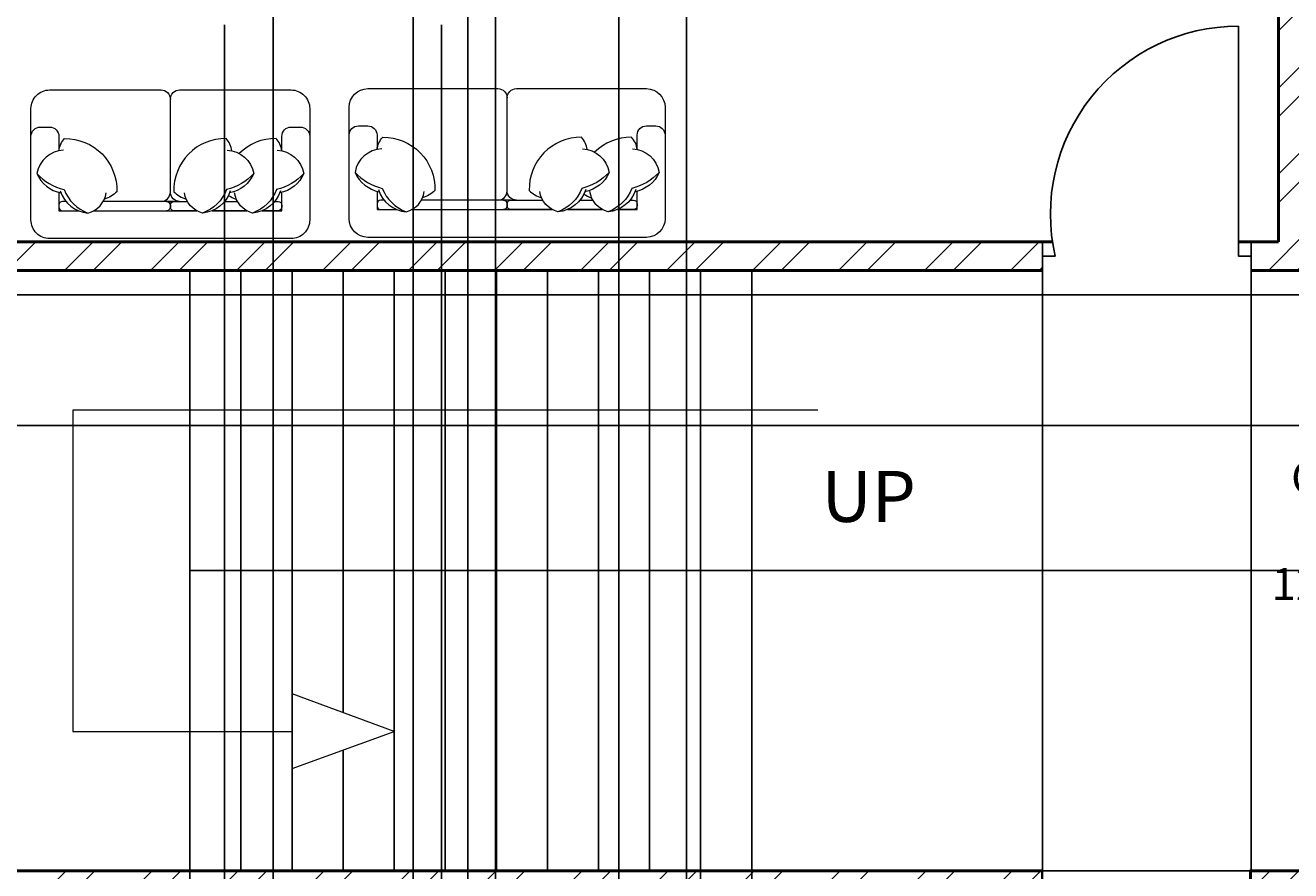
# Model space of a CAD drawing. Units: inches. Extents: x 2310 to 2937, y 1113 to 2410.
# Tile 8 of 23: x 2411 to 2609, y 2000 to 2132. Entities that reach past the tile are written whole.
import ezdxf

# ---------------------------------------------------------------- set-up
doc = ezdxf.new("R2010")
doc.units = ezdxf.units.IN
for name, color, linetype, lineweight in [('A-ANNO-DIMS', 2, 'Continuous', 18), ('A-ANNO-SYMB', 151, 'Continuous', 18), ('A-ANNO-TEXT', 7, 'Continuous', 18), ('A-AREA-IDEN', 7, 'Continuous', 18), ('A-DOOR', 31, 'Continuous', 25), ('A-FLOR-STRS', 151, 'Continuous', 25), ('A-FURN', 8, 'Continuous', 18), ('A-WALL', 7, 'Continuous', 50), ('A-WALL-PATT', 85, 'Continuous', 13)]:
    doc.layers.add(name, color=color, linetype=linetype, lineweight=lineweight)
doc.styles.get("Standard").update_dxf_attribs({"font": 'arial.ttf'})
doc.dimstyles.get("Standard").update_dxf_attribs({"dimtxt": 0.18, "dimasz": 0.18, "dimexe": 0.18, "dimexo": 0.0625, "dimgap": 0.09, "dimtad": 0, "dimtih": 1, "dimtoh": 1, "dimdec": 4, "dimzin": 0, "dimdsep": 46, "dimtxsty": 'Standard', "dimcen": 0.09, "dimadec": 0, "dimazin": 0, "dimtfac": 1, "dimtdec": 4, "dimtofl": 0, "dimtmove": 0, "dimatfit": 3, "dimfxl": 1, "dimtolj": 1, "dimtzin": 0, "dimarcsym": 0})

# ---------------------------------------------------------------- blocks, each defined once
blk = doc.blocks.new('SOFA-COMPACT')
at = {"ltscale": 0.03}
blk.add_lwpolyline([(20.37, 23.28, -0.414214), (21.83, 21.83, -0.414214), (23.28, 23.28), (40.75, 23.28, -0.414214), (43.66, 20.37), (43.66, 2.91, -0.414214), (40.75, 0), (2.91, 0, -0.414214), (0, 2.91), (0, 20.37, -0.414214), (2.91, 23.28), (20.37, 23.28, -0.414214), (21.83, 21.83, -0.414214), (23.28, 23.28)], format="xyb", dxfattribs=at)
for points in [[(20.37, 5.82, 0.414214), (21.83, 7.28), (21.83, 21.83, 0.414214)], [(23.28, 5.82, -0.414214), (21.83, 7.28), (21.83, 21.83, -0.414214)], [(0, 16.01, -0.414214), (1.46, 17.46), (2.91, 17.46, -0.414214), (4.37, 16.01), (4.37, 13.75)], [(39.29, 13.75), (39.29, 16.01, -0.414214), (40.75, 17.46), (42.2, 17.46, -0.414214), (43.66, 16.01)], [(4.36, 13.75, -0.165541), (5.26, 15.67, -0.425989), (13.44, 7.34, -0.121523), (11.5, 6.19, 7.115464)], [(31.45, 13.75, 0.165541), (30.55, 15.67, 0.425989), (22.38, 7.34, 0.121523), (24.32, 6.19, -7.115464)], [(39.29, 13.75, 0.165541), (38.39, 15.67, 0.200231), (32.62, 13.33, 0.121523)], [(5.1, 13.84, 0.356772), (0.93, 10.17, 0.249542), (4.7, 7.15, -9.61688)], [(30.72, 13.84, -0.356772), (34.89, 10.17, -0.249542), (31.11, 7.15, 9.61688)], [(38.56, 13.84, -0.356772), (42.73, 10.17, -0.249542), (38.95, 7.15, 9.61688)], [(0.93, 10.17, 0.14773), (5.18, 7.67, 0.213343), (8.93, 4, 0.178662)], [(34.89, 10.17, -0.14773), (30.64, 7.67, -0.213343), (26.88, 4, -0.178662)], [(42.73, 10.17, -0.14773), (38.48, 7.67, -0.213343), (34.72, 4, -0.178662)], [(4.59, 7.47, 0.306663), (8.93, 4, 0.30633), (11.77, 7.17, -0.872847)], [(20.37, 5.82, 0.414214), (21.83, 7.28)], [(23.28, 5.82, -0.414214), (21.83, 7.28)], [(31.22, 7.47, -0.306663), (26.88, 4, -0.30633), (24.05, 7.17, 0.872847)], [(30.94, 6.76, 0.071865), (32.16, 6.19, -7.115464)], [(39.06, 7.47, -0.306663), (34.72, 4, -0.30633), (31.89, 7.17, 0.872847)], [(36.23, 4.37), (39.29, 4.37), (39.29, 7.23, -0.414214)], [(5.48, 5.82), (4.95, 5.82, 0.414214), (4.37, 5.24), (4.37, 4.95, 0.414214), (4.95, 4.37)], [(4.95, 4.37), (7.43, 4.37, 0.414214)], [(9.85, 4.37), (21.25, 4.37, 0.414214), (21.83, 4.95), (21.83, 5.24, 0.414214), (21.25, 5.82), (11.31, 5.82, 0.414214)], [(25.97, 4.37), (22.41, 4.37, -0.414214), (21.83, 4.95), (21.83, 5.24, -0.414214), (22.41, 5.82), (24.5, 5.82, -0.414214)], [(33.81, 4.37), (28.39, 4.37, -0.414214)], [(30.34, 5.82), (32.34, 5.82, -0.414214)], [(38.71, 4.37), (36.23, 4.37, -0.414214)], [(38.18, 5.82), (38.71, 5.82, -0.414214), (39.29, 5.24), (39.29, 4.95, -0.414214), (38.71, 4.37)]]:
    blk.add_lwpolyline(points, format="xyb")
for points in [[(4.37, 7.23), (4.37, 4.37), (7.43, 4.37)], [(9.85, 4.37), (25.97, 4.37)], [(28.39, 4.37), (33.81, 4.37)]]:
    blk.add_lwpolyline(points)
blk.add_lwpolyline([(21.25, 4.37), (22.41, 4.37, -0.414214), (21.83, 4.95), (21.83, 5.24, -0.414214), (22.41, 5.82), (21.25, 5.82, -0.414214), (21.83, 5.24), (21.83, 4.95, -0.414214)], format="xyb", close=True)
blk = doc.blocks.new('*D41')
at = {"layer": 'A-ANNO-DIMS', "color": 0, "lineweight": -2, "transparency": 16777216}
for p, q in [((2479.99, 2347.45), (2479.99, 1649.5)), ((2503.66, 2347.45), (2503.66, 1649.5)), ((2480.17, 1649.68), (2491.36, 1649.68)), ((2503.48, 1649.68), (2492.29, 1649.68))]:
    blk.add_line(p, q, dxfattribs=at)
at = {"layer": 'A-ANNO-DIMS', "color": 0, "transparency": 16777216}
for points in [[(2480.17, 1649.71), (2480.17, 1649.65), (2479.99, 1649.68)], [(2503.48, 1649.71), (2503.48, 1649.65), (2503.66, 1649.68)]]:
    blk.add_solid(points, dxfattribs=at)
at = {"layer": 'Defpoints', "color": 0, "transparency": 16777216}
for p in [(2479.99, 2347.51), (2503.66, 2347.51), (2503.66, 1649.68)]:
    blk.add_point(p, dxfattribs=at)
at = {"layer": 'A-ANNO-DIMS', "color": 0, "transparency": 16777216, "insert": (2491.82, 1649.68), "char_height": 0.18, "attachment_point": 5}
blk.add_mtext('\\A1;23.676', dxfattribs=at)
blk = doc.blocks.new('*D60')
at = {"layer": 'A-ANNO-DIMS', "color": 0, "lineweight": -2, "transparency": 16777216}
for p, q in [((2449.5, 2205.95), (2449.5, 1649.5)), ((2471.44, 2205.95), (2471.44, 1649.5)), ((2449.68, 1649.68), (2460.01, 1649.68)), ((2471.26, 1649.68), (2460.94, 1649.68))]:
    blk.add_line(p, q, dxfattribs=at)
at = {"layer": 'A-ANNO-DIMS', "color": 0, "transparency": 16777216}
for points in [[(2449.68, 1649.71), (2449.68, 1649.65), (2449.5, 1649.68)], [(2471.26, 1649.71), (2471.26, 1649.65), (2471.44, 1649.68)]]:
    blk.add_solid(points, dxfattribs=at)
at = {"layer": 'Defpoints', "color": 0, "transparency": 16777216}
for p in [(2449.5, 2206.01), (2471.44, 2206.01), (2471.44, 1649.68)]:
    blk.add_point(p, dxfattribs=at)
at = {"layer": 'A-ANNO-DIMS', "color": 0, "transparency": 16777216, "insert": (2460.47, 1649.68), "char_height": 0.18, "attachment_point": 5}
blk.add_mtext('\\A1;21.936', dxfattribs=at)
blk = doc.blocks.new('*D61')
at = {"layer": 'A-ANNO-DIMS', "color": 0, "lineweight": -2, "transparency": 16777216}
for p, q in [((2484.33, 2205.95), (2484.33, 1649.5)), ((2514.27, 2205.95), (2514.27, 1649.5)), ((2484.51, 1649.68), (2498.9, 1649.68)), ((2514.09, 1649.68), (2499.69, 1649.68))]:
    blk.add_line(p, q, dxfattribs=at)
at = {"layer": 'A-ANNO-DIMS', "color": 0, "transparency": 16777216}
for points in [[(2484.51, 1649.71), (2484.51, 1649.65), (2484.33, 1649.68)], [(2514.09, 1649.71), (2514.09, 1649.65), (2514.27, 1649.68)]]:
    blk.add_solid(points, dxfattribs=at)
at = {"layer": 'Defpoints', "color": 0, "transparency": 16777216}
for p in [(2484.33, 2206.01), (2514.27, 2206.01), (2514.27, 1649.68)]:
    blk.add_point(p, dxfattribs=at)
at = {"layer": 'A-ANNO-DIMS', "color": 0, "transparency": 16777216, "insert": (2499.3, 1649.68), "char_height": 0.18, "attachment_point": 5}
blk.add_mtext('\\A1;29.94', dxfattribs=at)
blk = doc.blocks.new('*D62')
at = {"layer": 'A-ANNO-DIMS', "color": 0, "lineweight": -2, "transparency": 16777216}
for p, q in [((2569.99, 2093.45), (2569.99, 1649.5)), ((2602.69, 2093.45), (2602.69, 1649.5)), ((2570.17, 1649.68), (2586.02, 1649.68)), ((2602.51, 1649.68), (2586.66, 1649.68))]:
    blk.add_line(p, q, dxfattribs=at)
at = {"layer": 'A-ANNO-DIMS', "color": 0, "transparency": 16777216}
for points in [[(2570.17, 1649.71), (2570.17, 1649.65), (2569.99, 1649.68)], [(2602.51, 1649.71), (2602.51, 1649.65), (2602.69, 1649.68)]]:
    blk.add_solid(points, dxfattribs=at)
at = {"layer": 'Defpoints', "color": 0, "transparency": 16777216}
for p in [(2569.99, 2093.51), (2602.69, 2093.51), (2602.69, 1649.68)]:
    blk.add_point(p, dxfattribs=at)
at = {"layer": 'A-ANNO-DIMS', "color": 0, "transparency": 16777216, "insert": (2586.34, 1649.68), "char_height": 0.18, "attachment_point": 5}
blk.add_mtext('\\A1;32.7', dxfattribs=at)
blk = doc.blocks.new('*D64')
at = {"layer": 'A-ANNO-DIMS', "color": 0, "lineweight": -2, "transparency": 16777216}
for p, q in [((2524.527191, 2046.513944), (2858.015941, 2046.513944)), ((2857.835941, 2046.333944), (2857.835941, 2023.193944)), ((2857.835941, 1999.693944), (2857.835941, 2022.833944)), ((2524.527191, 1999.513944), (2858.015941, 1999.513944))]:
    blk.add_line(p, q, dxfattribs=at)
at = {"layer": 'A-ANNO-DIMS', "color": 0, "transparency": 16777216}
for points in [[(2857.805941, 2046.333944), (2857.865941, 2046.333944), (2857.835941, 2046.513944)], [(2857.805941, 1999.693944), (2857.865941, 1999.693944), (2857.835941, 1999.513944)]]:
    blk.add_solid(points, dxfattribs=at)
at = {"layer": 'Defpoints', "color": 0, "transparency": 16777216}
for p in [(2524.464691, 2046.513944), (2857.835941, 2046.513944), (2524.464691, 1999.513944)]:
    blk.add_point(p, dxfattribs=at)
at = {"layer": 'A-ANNO-DIMS', "color": 0, "transparency": 16777216, "insert": (2857.835941, 2023.013944), "char_height": 0.18, "attachment_point": 5}
blk.add_mtext('\\A1;47', dxfattribs=at)
blk = doc.blocks.new('*D65')
at = {"layer": 'A-ANNO-DIMS', "color": 0, "lineweight": -2, "transparency": 16777216}
for p, q in [((2403.49, 2093.45), (2403.49, 1649.5)), ((2436.46, 2093.45), (2436.46, 1649.5)), ((2403.67, 1649.68), (2419.58, 1649.68)), ((2436.28, 1649.68), (2420.37, 1649.68))]:
    blk.add_line(p, q, dxfattribs=at)
at = {"layer": 'A-ANNO-DIMS', "color": 0, "transparency": 16777216}
for points in [[(2403.67, 1649.71), (2403.67, 1649.65), (2403.49, 1649.68)], [(2436.28, 1649.71), (2436.28, 1649.65), (2436.46, 1649.68)]]:
    blk.add_solid(points, dxfattribs=at)
at = {"layer": 'Defpoints', "color": 0, "transparency": 16777216}
for p in [(2403.49, 2093.51), (2436.46, 2093.51), (2436.46, 1649.68)]:
    blk.add_point(p, dxfattribs=at)
at = {"layer": 'A-ANNO-DIMS', "color": 0, "transparency": 16777216, "insert": (2419.98, 1649.68), "char_height": 0.18, "attachment_point": 5}
blk.add_mtext('\\A1;32.98', dxfattribs=at)
blk = doc.blocks.new('*D66')
at = {"layer": 'A-ANNO-DIMS', "color": 0, "lineweight": -2, "transparency": 16777216}
for p, q in [((2516.46, 2093.45), (2516.46, 1649.5)), ((2524.46, 2093.45), (2524.46, 1649.5)), ((2516.64, 1649.68), (2520.32, 1649.68)), ((2524.28, 1649.68), (2520.61, 1649.68))]:
    blk.add_line(p, q, dxfattribs=at)
at = {"layer": 'A-ANNO-DIMS', "color": 0, "transparency": 16777216}
for points in [[(2516.64, 1649.71), (2516.64, 1649.65), (2516.46, 1649.68)], [(2524.28, 1649.71), (2524.28, 1649.65), (2524.46, 1649.68)]]:
    blk.add_solid(points, dxfattribs=at)
at = {"layer": 'Defpoints', "color": 0, "transparency": 16777216}
for p in [(2516.46, 2093.51), (2524.46, 2093.51), (2524.46, 1649.68)]:
    blk.add_point(p, dxfattribs=at)
at = {"layer": 'A-ANNO-DIMS', "color": 0, "transparency": 16777216, "insert": (2520.46, 1649.68), "char_height": 0.18, "attachment_point": 5}
blk.add_mtext('\\A1;8', dxfattribs=at)
blk = doc.blocks.new('*D67')
at = {"layer": 'A-ANNO-DIMS', "color": 0, "lineweight": -2, "transparency": 16777216}
for p, q in [((2684.42, 2089.69), (2360.46, 2089.69)), ((2360.64, 2089.51), (2360.64, 2079.64)), ((2360.64, 2069.41), (2360.64, 2079.28)), ((2684.42, 2069.23), (2360.46, 2069.23))]:
    blk.add_line(p, q, dxfattribs=at)
at = {"layer": 'A-ANNO-DIMS', "color": 0, "transparency": 16777216}
for points in [[(2360.61, 2089.51), (2360.67, 2089.51), (2360.64, 2089.69)], [(2360.61, 2069.41), (2360.67, 2069.41), (2360.64, 2069.23)]]:
    blk.add_solid(points, dxfattribs=at)
at = {"layer": 'Defpoints', "color": 0, "transparency": 16777216}
for p in [(2360.64, 2089.69), (2684.49, 2089.69), (2684.49, 2069.23)]:
    blk.add_point(p, dxfattribs=at)
at = {"layer": 'A-ANNO-DIMS', "color": 0, "transparency": 16777216, "insert": (2360.64, 2079.46), "char_height": 0.18, "attachment_point": 5}
blk.add_mtext('\\A1;20.46', dxfattribs=at)
blk = doc.blocks.new('*D69')
at = {"layer": 'A-ANNO-DIMS', "color": 0, "lineweight": -2, "transparency": 16777216}
for p, q in [((2441.86, 2131.96), (2441.86, 1649.5)), ((2475.89, 2131.96), (2475.89, 1649.5)), ((2442.04, 1649.68), (2458.48, 1649.68)), ((2475.71, 1649.68), (2459.27, 1649.68))]:
    blk.add_line(p, q, dxfattribs=at)
at = {"layer": 'A-ANNO-DIMS', "color": 0, "transparency": 16777216}
for points in [[(2442.04, 1649.71), (2442.04, 1649.65), (2441.86, 1649.68)], [(2475.71, 1649.71), (2475.71, 1649.65), (2475.89, 1649.68)]]:
    blk.add_solid(points, dxfattribs=at)
at = {"layer": 'Defpoints', "color": 0, "transparency": 16777216}
for p in [(2441.86, 2132.02), (2475.89, 2132.02), (2475.89, 1649.68)]:
    blk.add_point(p, dxfattribs=at)
at = {"layer": 'A-ANNO-DIMS', "color": 0, "transparency": 16777216, "insert": (2458.88, 1649.68), "char_height": 0.18, "attachment_point": 5}
blk.add_mtext('\\A1;34.03', dxfattribs=at)

msp = doc.modelspace()

# ---------------------------------------------------------------- hatches: boundary and pattern name
at = {"layer": 'A-WALL-PATT'}
h = msp.add_hatch(dxfattribs=at)
h.set_pattern_fill('ANSI32', color=256)
h.paths.add_polyline_path([(2639.1394, 2356.5139), (2563.662, 2356.5139), (2563.662, 2347.5139), (2606.9859, 2347.5139), (2606.9859, 2210.5139), (2514.2692, 2210.5139), (2514.2692, 2206.0139), (2606.9859, 2206.0139), (2606.9859, 2098.0139), (2602.689, 2098.0139), (2602.689, 2093.5139), (2615.5262, 2093.5139), (2615.5262, 2095.7639), (2615.5262, 2098.0139), (2611.4859, 2098.0139), (2611.4859, 2206.0139), (2703.9391, 2206.0139), (2703.9391, 2208.2639), (2703.9391, 2210.5139), (2611.4859, 2210.5139), (2611.4859, 2347.5139), (2639.1394, 2347.5139)])
h.paths.add_polyline_path([(2823.9859, 2356.5139), (2699.1394, 2356.5139), (2699.1394, 2347.5139), (2738.4859, 2347.5139), (2738.4859, 2343.9266), (2742.9859, 2343.9266), (2742.9859, 2347.5139), (2814.9859, 2347.5139), (2814.9859, 2336.76), (2823.9859, 2336.76)])
h.paths.add_polyline_path([(2823.9859, 2312.76), (2814.9859, 2312.76), (2814.9859, 2299.5139), (2742.9859, 2299.5139), (2742.9859, 2323.0159), (2740.7359, 2323.0159), (2738.4859, 2323.0159), (2738.4859, 2210.5139), (2734.5483, 2210.5139), (2734.5483, 2206.0139), (2746.8769, 2206.0139), (2746.8769, 2208.2639), (2746.8769, 2210.5139), (2742.9859, 2210.5139), (2742.9859, 2295.0139), (2814.9859, 2295.0139), (2814.9859, 2269.8977), (2823.9859, 2269.8977)])
h.paths.add_polyline_path([(2823.9859, 2210.5139), (2823.9859, 2233.8977), (2819.4859, 2233.8977), (2814.9859, 2233.8977), (2814.9859, 2210.5139), (2769.9745, 2210.5139), (2769.9745, 2206.0139), (2814.9859, 2206.0139), (2814.9859, 2178.3027), (2823.9859, 2178.3027)])
h.paths.add_polyline_path([(2823.9859, 2118.3027), (2819.4859, 2118.3027), (2814.9859, 2118.3027), (2814.9859, 2098.0139), (2647.0333, 2098.0139), (2647.0333, 2093.5139), (2814.9859, 2093.5139), (2814.9859, 1999.5139), (2650.6052, 1999.5139), (2650.6052, 1995.0139), (2814.9859, 1995.0139), (2814.9859, 1969.9784), (2823.9859, 1969.9784)])
h.paths.add_polyline_path([(2403.4859, 2093.5139), (2569.9888, 2093.5139), (2569.9888, 2095.7639), (2569.9888, 2098.0139), (2403.4859, 2098.0139), (2403.4859, 2131.7587), (2394.4859, 2131.7587), (2394.4859, 1967.522), (2403.4859, 1967.522), (2403.4859, 1995.0139), (2569.8903, 1995.0139), (2569.8903, 1997.2639), (2569.8903, 1999.5139), (2403.4859, 1999.5139)])
h.paths.add_polyline_path([(2503.662, 2356.5139), (2394.4859, 2356.5139), (2394.4859, 2337.9231), (2398.9859, 2337.9231), (2403.4859, 2337.9231), (2403.4859, 2347.5139), (2475.4859, 2347.5139), (2475.4859, 2343.0384), (2479.9859, 2343.0384), (2479.9859, 2347.5139), (2503.662, 2347.5139)])
h.paths.add_polyline_path([(2498.3065, 1745.5139), (2479.9859, 1745.5139), (2479.9859, 1749.1663), (2477.7359, 1749.1663), (2475.4859, 1749.1663), (2475.4859, 1745.5139), (2403.4859, 1745.5139), (2403.4859, 1753.6409), (2398.9859, 1753.6409), (2394.4859, 1753.6409), (2394.4859, 1736.5139), (2498.3065, 1736.5139), (2498.3065, 1741.0139)])
h.paths.add_polyline_path([(2479.9859, 1882.5139), (2483.9367, 1882.5139), (2483.9367, 1887.0139), (2471.5501, 1887.0139), (2471.5501, 1885.1969), (2471.5501, 1882.5139), (2475.4859, 1882.5139), (2475.4859, 1798.0139), (2403.4859, 1798.0139), (2403.4859, 1828.0433), (2402.2852, 1828.0433), (2394.4859, 1828.0433), (2394.4859, 1777.6409), (2403.4859, 1777.6409), (2403.4859, 1793.5139), (2475.4859, 1793.5139), (2475.4859, 1769.1696), (2479.9859, 1769.1696)])
h.paths.add_polyline_path([(2403.4859, 1907.522), (2398.9859, 1907.522), (2394.4859, 1907.522), (2394.4859, 1864.0433), (2403.4859, 1864.0433), (2403.4859, 1882.5139), (2448.9325, 1882.5139), (2448.9325, 1884.7639), (2448.9325, 1887.0139), (2403.4859, 1887.0139)])
h.paths.add_polyline_path([(2702.2061, 1887.0139), (2611.4859, 1887.0139), (2611.4859, 1995.0139), (2615.6132, 1995.0139), (2615.6132, 1999.5139), (2602.4798, 1999.5139), (2602.4798, 1997.2639), (2602.4798, 1995.0139), (2606.9859, 1995.0139), (2606.9859, 1887.0139), (2516.2443, 1887.0139), (2516.2443, 1884.7639), (2516.2443, 1882.5139), (2606.9859, 1882.5139), (2606.9859, 1745.5139), (2558.3065, 1745.5139), (2558.3065, 1736.5139), (2638.8921, 1736.5139), (2638.8921, 1741.0139), (2638.8921, 1745.5139), (2611.4859, 1745.5139), (2611.4859, 1882.5139), (2702.2061, 1882.5139)])
h.paths.add_polyline_path([(2823.9859, 1909.9784), (2819.4859, 1909.9784), (2814.9859, 1909.9784), (2814.9859, 1887.0139), (2769.144, 1887.0139), (2769.144, 1884.7639), (2769.144, 1882.5139), (2814.9859, 1882.5139), (2814.9859, 1854.1704), (2823.9859, 1854.1704)])
h.paths.add_polyline_path([(2823.9859, 1818.1704), (2819.4859, 1818.1704), (2814.9859, 1818.1704), (2814.9859, 1798.0139), (2742.9859, 1798.0139), (2742.9859, 1882.5139), (2746.805, 1882.5139), (2746.805, 1887.0139), (2733.7334, 1887.0139), (2733.7334, 1884.7639), (2733.7334, 1882.5139), (2738.4859, 1882.5139), (2738.4859, 1771.1728), (2740.7359, 1771.1728), (2742.9859, 1771.1728), (2742.9859, 1793.5139), (2814.9859, 1793.5139), (2814.9859, 1783.6684), (2823.9859, 1783.6684)])
h.paths.add_polyline_path([(2823.9859, 1759.6684), (2814.9859, 1759.6684), (2814.9859, 1745.5139), (2742.9859, 1745.5139), (2742.9859, 1748.9831), (2740.7359, 1748.9831), (2738.4859, 1748.9831), (2738.4859, 1745.5139), (2698.8921, 1745.5139), (2698.8921, 1736.5139), (2823.9859, 1736.5139)])

# ---------------------------------------------------------------- linework, layer by layer
at = {"layer": 'A-ANNO-SYMB'}
for p, q in [((2534.8253, 2071.6394), (2418.1256, 2071.6394)), ((2418.1256, 2071.6394), (2418.1256, 2021.3291)), ((2468.4647, 2021.3291), (2452.4647, 2027.221)), ((2452.4647, 2027.221), (2452.4647, 2015.5057)), ((2418.1256, 2021.3291), (2452.4647, 2021.3291)), ((2452.4647, 2015.5057), (2468.4647, 2021.3291))]:
    msp.add_line(p, q, dxfattribs=at)
at = {"layer": 'A-DOOR'}
for p, q in [((2600.689, 2095.7639), (2600.689, 2131.7639)), ((2569.9888, 2098.0139), (2569.9888, 2093.5139)), ((2602.689, 2098.0139), (2602.689, 2093.5139)), ((2569.9888, 2093.5139), (2569.9888, 2095.7639)), ((2569.9888, 2095.7639), (2571.9888, 2095.7639)), ((2602.689, 2095.7639), (2600.689, 2095.7639)), ((2602.689, 2093.5139), (2602.689, 2095.7639)), ((2569.8903, 1999.5139), (2569.8903, 1995.0139)), ((2602.4798, 1995.0139), (2602.4798, 1999.5139)), ((2602.4798, 1999.5139), (2602.4798, 1997.2639))]:
    msp.add_line(p, q, dxfattribs=at)
msp.add_arc((2600.689, 2102.3236), 29.4403, 90, 192.874238, dxfattribs=at)
at = {"layer": 'A-FLOR-STRS'}
for p, q in [((2436.4647, 2093.5139), (2436.4647, 1999.5139)), ((2444.4647, 2093.5139), (2444.4647, 1999.5139)), ((2452.4647, 2093.5139), (2452.4647, 1999.5139)), ((2460.4647, 2093.5139), (2460.4647, 2024.2751)), ((2468.4647, 2093.5139), (2468.4647, 1999.5139)), ((2476.4647, 2093.5139), (2476.4647, 1999.5139)), ((2484.4647, 2093.5139), (2484.4647, 1999.5139)), ((2492.4647, 2093.5139), (2492.4647, 1999.5139)), ((2500.4647, 2093.5139), (2500.4647, 1999.5139)), ((2508.4647, 2093.5139), (2508.4647, 1999.5139)), ((2516.4647, 2093.5139), (2516.4647, 1999.5139)), ((2524.4647, 2093.5139), (2524.4647, 1999.5139)), ((2436.4647, 1999.5139), (2436.4647, 2046.5139)), ((2436.4647, 2046.5139), (2524.4647, 2046.5139)), ((2460.4647, 2018.4174), (2460.4647, 1999.5139))]:
    msp.add_line(p, q, dxfattribs=at)
at = {"layer": 'A-FURN', "ltscale": 0.03}
msp.add_lwpolyline([(2484.6976, 2121.9757, -0.41421356), (2486.1528, 2120.5205, -0.41421356), (2487.608, 2121.9757), (2507.9806, 2121.9757, -0.41421356), (2510.891, 2119.0653), (2510.891, 2101.603, -0.41421356), (2507.9806, 2098.6927), (2464.325, 2098.6927, -0.41421356), (2461.4146, 2101.603), (2461.4146, 2119.0653, -0.41421356), (2464.325, 2121.9757), (2484.6976, 2121.9757, -0.41421356), (2486.1528, 2120.5205, -0.41421356), (2487.608, 2121.9757)], format="xyb", dxfattribs=at)
at = {"layer": 'A-FURN'}
for points in [[(2484.6976, 2104.5134, 0.41421356), (2486.1528, 2105.9686), (2486.1528, 2120.5205, 0.41421356)], [(2487.608, 2104.5134, -0.41421356), (2486.1528, 2105.9686), (2486.1528, 2120.5205, -0.41421356)], [(2461.4146, 2114.6997, -0.41421356), (2462.8698, 2116.1549), (2464.325, 2116.1549, -0.41421356), (2465.7802, 2114.6997), (2465.7802, 2112.4451)], [(2506.5255, 2112.4451), (2506.5255, 2114.6997, -0.41421356), (2507.9806, 2116.1549), (2509.4358, 2116.1549, -0.41421356), (2510.891, 2114.6997)], [(2465.777, 2112.4445, -0.16554063), (2466.6772, 2114.3672, -0.42598917), (2474.8499, 2106.0309, -0.12152332), (2472.9098, 2104.8819, 7.11546429)], [(2498.6896, 2112.4445, 0.16554063), (2497.7893, 2114.3672, 0.42598917), (2489.6167, 2106.0309, 0.12152332), (2491.5568, 2104.8819, -7.11546429)], [(2506.5286, 2112.4445, 0.16554063), (2505.6284, 2114.3672, 0.20023115), (2499.8518, 2112.0255, 0.12152332)], [(2466.5104, 2112.5332, 0.35677236), (2462.3407, 2108.8652, 0.24954205), (2466.1189, 2105.8425, -9.61688035)], [(2497.9561, 2112.5332, -0.35677236), (2502.1258, 2108.8652, -0.24954205), (2498.3477, 2105.8425, 9.61688035)], [(2505.7952, 2112.5332, -0.35677236), (2509.9649, 2108.8652, -0.24954205), (2506.1868, 2105.8425, 9.61688035)], [(2462.3407, 2108.8652, 0.14772988), (2466.5938, 2106.3643, 0.21334276), (2470.3466, 2102.6964, 0.17866181)], [(2502.1258, 2108.8652, -0.14772988), (2497.8727, 2106.3643, -0.21334276), (2494.12, 2102.6964, -0.17866181)], [(2509.9649, 2108.8652, -0.14772988), (2505.7118, 2106.3643, -0.21334276), (2501.9591, 2102.6964, -0.17866181)], [(2466.0063, 2106.165, 0.30666349), (2470.3466, 2102.6964, 0.30632997), (2473.182, 2105.8641, -0.87284716)], [(2484.6976, 2104.5134, 0.41421356), (2486.1528, 2105.9686)], [(2487.608, 2104.5134, -0.41421356), (2486.1528, 2105.9686)], [(2498.4603, 2106.165, -0.30666349), (2494.12, 2102.6964, -0.30632997), (2491.2846, 2105.8641, 0.87284716)], [(2498.1758, 2105.4508, 0.07186538), (2499.3958, 2104.8819, -7.11546429)], [(2506.2994, 2106.165, -0.30666349), (2501.9591, 2102.6964, -0.30632997), (2499.1237, 2105.8641, 0.87284716)], [(2503.4641, 2103.0582), (2506.5255, 2103.0582), (2506.5255, 2105.918, -0.41421356)], [(2466.8906, 2104.5134), (2466.3622, 2104.5134, 0.41421356), (2465.7802, 2103.9313), (2465.7802, 2103.6403, 0.41421356), (2466.3622, 2103.0582)], [(2466.3622, 2103.0582), (2468.8415, 2103.0582, 0.41421356)], [(2471.2624, 2103.0582), (2485.5707, 2103.0582, 0.41421356), (2486.1528, 2103.6403), (2486.1528, 2103.9313, 0.41421356), (2485.5707, 2104.5134), (2472.7277, 2104.5134, 0.41421356)], [(2493.2042, 2103.0582), (2486.7349, 2103.0582, -0.41421356), (2486.1528, 2103.6403), (2486.1528, 2103.9313, -0.41421356), (2486.7349, 2104.5134), (2491.7389, 2104.5134, -0.41421356)], [(2501.0432, 2103.0582), (2495.6251, 2103.0582, -0.41421356)], [(2497.5759, 2104.5134), (2499.5779, 2104.5134, -0.41421356)], [(2505.9434, 2103.0582), (2503.4641, 2103.0582, -0.41421356)], [(2505.415, 2104.5134), (2505.9434, 2104.5134, -0.41421356), (2506.5255, 2103.9313), (2506.5255, 2103.6403, -0.41421356), (2505.9434, 2103.0582)]]:
    msp.add_lwpolyline(points, format="xyb", dxfattribs=at)
for points in [[(2465.7802, 2105.918), (2465.7802, 2103.0582), (2468.8415, 2103.0582)], [(2471.2624, 2103.0582), (2493.2042, 2103.0582)], [(2495.6251, 2103.0582), (2501.0432, 2103.0582)]]:
    msp.add_lwpolyline(points, dxfattribs=at)
msp.add_lwpolyline([(2485.5707, 2103.0582), (2486.7349, 2103.0582, -0.41421356), (2486.1528, 2103.6403), (2486.1528, 2103.9313, -0.41421356), (2486.7349, 2104.5134), (2485.5707, 2104.5134, -0.41421356), (2486.1528, 2103.9313), (2486.1528, 2103.6403, -0.41421356)], format="xyb", close=True, dxfattribs=at)
at = {"layer": 'A-WALL'}
for p, q in [((2606.9859, 2206.0139), (2606.9859, 2098.0139)), ((2403.4859, 2098.0139), (2571.5658, 2098.0139)), ((2600.689, 2098.0139), (2606.9859, 2098.0139)), ((2403.4859, 2093.5139), (2569.9888, 2093.5139)), ((2602.689, 2093.5139), (2615.5262, 2093.5139)), ((2403.4859, 1999.5139), (2569.8903, 1999.5139)), ((2602.4798, 1999.5139), (2615.6132, 1999.5139))]:
    msp.add_line(p, q, dxfattribs=at)

# ---------------------------------------------------------------- block references
at = {"layer": 'A-FURN'}
msp.add_blockref('SOFA-COMPACT', (2411.5736, 2098.4972), dxfattribs=at)

# ---------------------------------------------------------------- texts
at = {"layer": 'A-ANNO-TEXT', "insert": (2535.3995, 2062.1234), "char_height": 8, "attachment_point": 1}
msp.add_mtext_dynamic_manual_height_columns('UP', width=40.064141, gutter_width=12.5, heights=[0], dxfattribs=at)
at = {"layer": 'A-AREA-IDEN', "insert": (2598.2625, 2063.5751), "char_height": 5, "attachment_point": 1}
msp.add_mtext_dynamic_manual_height_columns('       COMMON\\P        LOBBY\\P     12\'2"x7\'10"', width=93.589377, gutter_width=12.5, heights=[0], dxfattribs=at)

# ---------------------------------------------------------------- dimensions: what is measured, and where the dimension line sits
at = {"layer": 'A-ANNO-DIMS'}
for base, p1, p2, override, picture, middle in [((2503.662, 1649.6807), (2479.9859, 2347.5139), (2503.662, 2347.5139), {"dimdec": 3, "dimlfac": 1, "dimrnd": 0, "dimzin": 0, "dimdsep": 46, "dimlunit": 2}, '*D41', (2491.824, 1649.6807)), ((2471.4388, 1649.6807), (2449.5024, 2206.0139), (2471.4388, 2206.0139), {"dimdec": 3, "dimlfac": 1, "dimrnd": 0, "dimzin": 0, "dimdsep": 46, "dimlunit": 2}, '*D60', (2460.4706, 1649.6807)), ((2514.2692, 1649.6807), (2484.3278, 2206.0139), (2514.2692, 2206.0139), {"dimdec": 2, "dimlfac": 1, "dimrnd": 0, "dimzin": 0, "dimdsep": 46, "dimlunit": 2}, '*D61', (2499.2985, 1649.6807)), ((2475.8929, 1649.6807), (2441.8613, 2132.0241), (2475.8929, 2132.0241), {"dimdec": 2, "dimlfac": 1, "dimrnd": 0, "dimzin": 0, "dimdsep": 46, "dimlunit": 2}, '*D69', (2458.8771, 1649.6807)), ((2436.4647, 1649.6807), (2403.4859, 2093.5139), (2436.4647, 2093.5139), {"dimdec": 2, "dimlfac": 1, "dimrnd": 0, "dimzin": 0, "dimdsep": 46, "dimlunit": 2}, '*D65', (2419.9753, 1649.6807)), ((2524.4647, 1649.6807), (2516.4647, 2093.5139), (2524.4647, 2093.5139), {"dimdec": 0, "dimlfac": 1, "dimrnd": 0, "dimzin": 0, "dimdsep": 46, "dimlunit": 2}, '*D66', (2520.4647, 1649.6807)), ((2602.689, 1649.6807), (2569.9888, 2093.5139), (2602.689, 2093.5139), {"dimdec": 1, "dimlfac": 1, "dimrnd": 0, "dimzin": 0, "dimdsep": 46, "dimlunit": 2}, '*D62', (2586.3389, 1649.6807))]:
    dim = msp.add_linear_dim(base=base, p1=p1, p2=p2, dimstyle='Standard', override=override, dxfattribs=at)
    dim.commit()
    dim.dimension.update_dxf_attribs({"geometry": picture, "text_midpoint": middle})
for base, p1, p2, override, picture, middle in [((2360.6359, 2089.6861), (2684.4859, 2069.228), (2684.4859, 2089.6861), {"dimdec": 2, "dimlfac": 1, "dimrnd": 0, "dimzin": 0, "dimdsep": 46, "dimlunit": 2}, '*D67', (2360.6359, 2079.457)), ((2857.8359, 2046.5139), (2524.4647, 1999.5139), (2524.4647, 2046.5139), {"dimdec": 0, "dimlfac": 1, "dimrnd": 0, "dimzin": 0, "dimdsep": 46, "dimlunit": 2}, '*D64', (2857.8359, 2023.0139))]:
    dim = msp.add_linear_dim(base=base, p1=p1, p2=p2, angle=90, dimstyle='Standard', override=override, dxfattribs=at)
    dim.commit()
    dim.dimension.update_dxf_attribs({"geometry": picture, "text_midpoint": middle})

doc.saveas('drawing.dxf')
